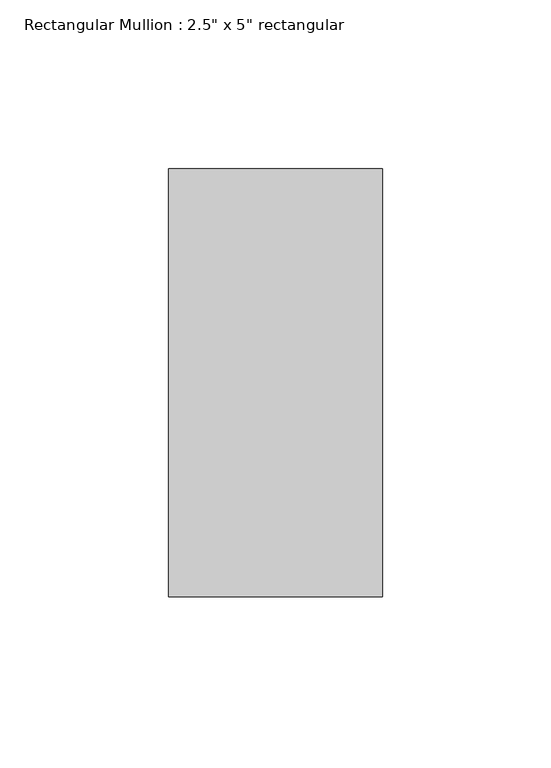
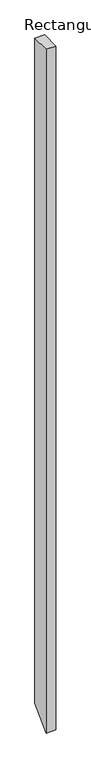
"""IFC4 building model written with IfcOpenShell, lengths in millimetres: member geometry."""

from ifc_helpers import new_model, si_unit, frame, origin, place, context, project, spatial, polyline, outline, extrude, source, transform, mapped, element, save


def member_5882a209(model_context):
    return source(origin(), model_context, "Body", "SweptSolid", [
        extrude(outline(polyline([(-63.5, 0.0), (63.5, 0.0), (63.5, -4582.7904401), (-63.5, -4709.7904401), (-63.5, 0.0)])), frame((-63.5, 0.0, 0.0), z_axis=(1.0, 0.0, 0.0), x_axis=(0.0, 1.0, 0.0)), (0.0, 0.0, 1.0), 63.5),
    ])


if __name__ == "__main__":
    model = new_model("IFC4")
    model_context = context("Model", 3, world=origin())
    ifc_project = project(units=[si_unit("LENGTHUNIT", "METRE", prefix="MILLI")], contexts=[model_context])
    site = spatial("IfcSite", under=ifc_project)
    building = spatial("IfcBuilding", under=site)
    placement = place(None, origin())
    member_shape = member_5882a209(model_context)
    element("IfcMember", 1, ObjectType="Rectangular Mullion : 2.5\" x 5\" rectangular", at=placement, inside=building, context=model_context, shape_type="MappedRepresentation", body=[
        mapped(member_shape, transform((0.0, 0.0, 0.0), x_axis=(1.0, 0.0, 0.0), y_axis=(0.0, 1.0, 0.0), z_axis=(0.0, 0.0, 1.0))),
    ])
    save(model, "model.ifc")

# Revit data of these elements
# Type "Rectangular Mullion : 2.5\" x 5\" rectangular"
#   built-in parameter 1007304 = 0.416667 (stored number, unit not read)
#   built-in parameter 1007301 = 0.104167 (stored number, unit not read)
#   built-in parameter 1007300 = 0.104167 (stored number, unit not read)
# Element 1 (IfcMember, "Rectangular Mullion : 2.5\" x 5\" rectangular")
#   Materials on its faces: "Aluminum"
# Materials
#   "Aluminum": class "Metal", colour RGB 247 247 247, transparency 0, Description = "Aluminum 6061", Cost = 0
